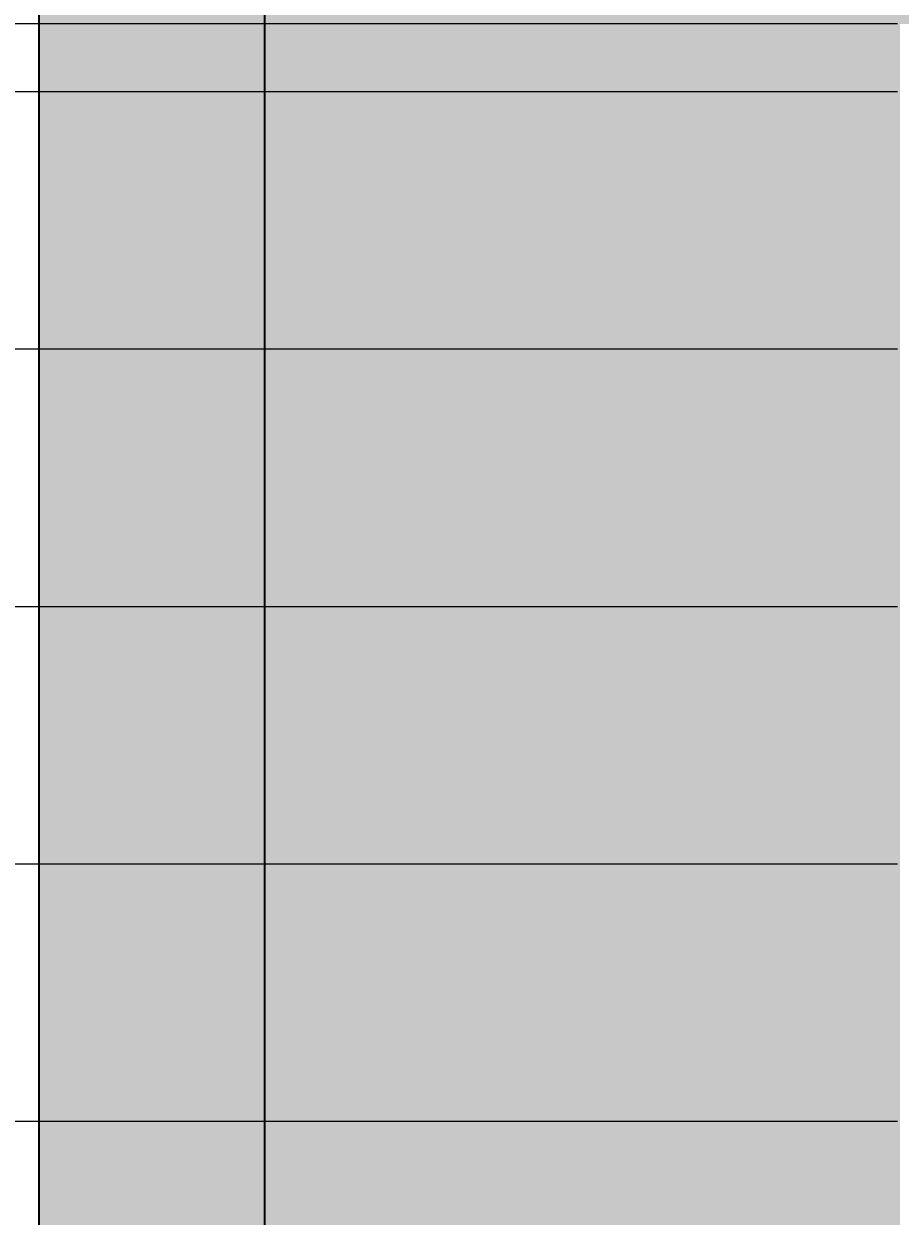
# Model space of a CAD drawing. Units: feet. Extents: x 2695 to 2912, y 795 to 1139.
# Tile 43 of 83: x 2710 to 2731, y 1020 to 1048. Entities that reach past the tile are written whole.
import ezdxf

# ---------------------------------------------------------------- set-up
doc = ezdxf.new("R2010")
doc.units = ezdxf.units.FT
for name, color, linetype, lineweight in [('A-ANNO-DIMS', 2, 'Continuous', 18), ('A-ELEV', 7, 'Continuous', 35), ('A-ELEV-PATT', 252, 'Continuous', 13)]:
    doc.layers.add(name, color=color, linetype=linetype, lineweight=lineweight)
doc.styles.get("Standard").update_dxf_attribs({"font": 'arial.ttf'})
doc.dimstyles.get("Standard").update_dxf_attribs({"dimtxt": 0.18, "dimasz": 0.18, "dimexe": 0.18, "dimexo": 0.0625, "dimgap": 0.09, "dimtad": 0, "dimtih": 1, "dimtoh": 1, "dimdec": 1, "dimzin": 0, "dimdsep": 46, "dimlunit": 3, "dimtxsty": 'Standard', "dimcen": 0.09, "dimadec": 0, "dimazin": 0, "dimtfac": 1, "dimtdec": 1, "dimtofl": 0, "dimtmove": 0, "dimatfit": 3, "dimfxl": 1, "dimtolj": 1, "dimtzin": 0, "dimarcsym": 0})

# ---------------------------------------------------------------- blocks, each defined once
blk = doc.blocks.new('*D12')
at = {"layer": 'A-ANNO-DIMS', "color": 0, "lineweight": -2, "transparency": 16777216}
for p, q in [((2710.574, 1122.931), (2694.681, 1122.931)), ((2694.861, 1122.751), (2694.861, 967.113)), ((2694.861, 811.111), (2694.861, 966.749)), ((2710.574, 810.931), (2694.681, 810.931))]:
    blk.add_line(p, q, dxfattribs=at)
at = {"layer": 'A-ANNO-DIMS', "color": 0, "transparency": 16777216}
for points in [[(2694.831, 1122.751), (2694.891, 1122.751), (2694.861, 1122.931)], [(2694.831, 811.111), (2694.891, 811.111), (2694.861, 810.931)]]:
    blk.add_solid(points, dxfattribs=at)
at = {"layer": 'Defpoints', "color": 0, "transparency": 16777216}
for p in [(2694.861, 1122.931), (2710.636, 1122.931), (2710.636, 810.931)]:
    blk.add_point(p, dxfattribs=at)
at = {"layer": 'A-ANNO-DIMS', "color": 0, "transparency": 16777216, "insert": (2694.861, 966.931), "char_height": 0.18, "attachment_point": 5}
blk.add_mtext('\\A1;312', dxfattribs=at)
blk = doc.blocks.new('*D41')
at = {"layer": 'A-ANNO-DIMS', "color": 0, "lineweight": -2, "transparency": 16777216}
for p, q in [((2730.646, 1022.518), (2694.681, 1022.518)), ((2694.861, 1022.338), (2694.861, 1019.7)), ((2694.861, 1016.698), (2694.861, 1019.336)), ((2730.646, 1016.518), (2694.681, 1016.518))]:
    blk.add_line(p, q, dxfattribs=at)
at = {"layer": 'A-ANNO-DIMS', "color": 0, "transparency": 16777216}
for points in [[(2694.831, 1022.338), (2694.891, 1022.338), (2694.861, 1022.518)], [(2694.831, 1016.698), (2694.891, 1016.698), (2694.861, 1016.518)]]:
    blk.add_solid(points, dxfattribs=at)
at = {"layer": 'Defpoints', "color": 0, "transparency": 16777216}
for p in [(2694.861, 1022.518), (2730.708, 1022.518), (2730.708, 1016.518)]:
    blk.add_point(p, dxfattribs=at)
at = {"layer": 'A-ANNO-DIMS', "color": 0, "transparency": 16777216, "insert": (2694.861, 1019.518), "char_height": 0.18, "attachment_point": 5}
blk.add_mtext('\\A1;6', dxfattribs=at)
blk = doc.blocks.new('*D42')
at = {"layer": 'A-ANNO-DIMS', "color": 0, "lineweight": -2, "transparency": 16777216}
for p, q in [((2730.646, 1028.518), (2694.681, 1028.518)), ((2694.861, 1028.338), (2694.861, 1025.7)), ((2694.861, 1022.698), (2694.861, 1025.336)), ((2730.646, 1022.518), (2694.681, 1022.518))]:
    blk.add_line(p, q, dxfattribs=at)
at = {"layer": 'A-ANNO-DIMS', "color": 0, "transparency": 16777216}
for points in [[(2694.831, 1028.338), (2694.891, 1028.338), (2694.861, 1028.518)], [(2694.831, 1022.698), (2694.891, 1022.698), (2694.861, 1022.518)]]:
    blk.add_solid(points, dxfattribs=at)
at = {"layer": 'Defpoints', "color": 0, "transparency": 16777216}
for p in [(2694.861, 1028.518), (2730.708, 1028.518), (2730.708, 1022.518)]:
    blk.add_point(p, dxfattribs=at)
at = {"layer": 'A-ANNO-DIMS', "color": 0, "transparency": 16777216, "insert": (2694.861, 1025.518), "char_height": 0.18, "attachment_point": 5}
blk.add_mtext('\\A1;6', dxfattribs=at)
blk = doc.blocks.new('*D43')
at = {"layer": 'A-ANNO-DIMS', "color": 0, "lineweight": -2, "transparency": 16777216}
for p, q in [((2730.646, 1034.518), (2694.681, 1034.518)), ((2694.861, 1034.338), (2694.861, 1031.7)), ((2694.861, 1028.698), (2694.861, 1031.336)), ((2730.646, 1028.518), (2694.681, 1028.518))]:
    blk.add_line(p, q, dxfattribs=at)
at = {"layer": 'A-ANNO-DIMS', "color": 0, "transparency": 16777216}
for points in [[(2694.831, 1034.338), (2694.891, 1034.338), (2694.861, 1034.518)], [(2694.831, 1028.698), (2694.891, 1028.698), (2694.861, 1028.518)]]:
    blk.add_solid(points, dxfattribs=at)
at = {"layer": 'Defpoints', "color": 0, "transparency": 16777216}
for p in [(2694.861, 1034.518), (2730.708, 1034.518), (2730.708, 1028.518)]:
    blk.add_point(p, dxfattribs=at)
at = {"layer": 'A-ANNO-DIMS', "color": 0, "transparency": 16777216, "insert": (2694.861, 1031.518), "char_height": 0.18, "attachment_point": 5}
blk.add_mtext('\\A1;6', dxfattribs=at)
blk = doc.blocks.new('*D44')
at = {"layer": 'A-ANNO-DIMS', "color": 0, "lineweight": -2, "transparency": 16777216}
for p, q in [((2730.646, 1040.518), (2694.681, 1040.518)), ((2694.861, 1040.338), (2694.861, 1037.7)), ((2694.861, 1034.698), (2694.861, 1037.336)), ((2730.646, 1034.518), (2694.681, 1034.518))]:
    blk.add_line(p, q, dxfattribs=at)
at = {"layer": 'A-ANNO-DIMS', "color": 0, "transparency": 16777216}
for points in [[(2694.831, 1040.338), (2694.891, 1040.338), (2694.861, 1040.518)], [(2694.831, 1034.698), (2694.891, 1034.698), (2694.861, 1034.518)]]:
    blk.add_solid(points, dxfattribs=at)
at = {"layer": 'Defpoints', "color": 0, "transparency": 16777216}
for p in [(2694.861, 1040.518), (2730.708, 1040.518), (2730.708, 1034.518)]:
    blk.add_point(p, dxfattribs=at)
at = {"layer": 'A-ANNO-DIMS', "color": 0, "transparency": 16777216, "insert": (2694.861, 1037.518), "char_height": 0.18, "attachment_point": 5}
blk.add_mtext('\\A1;6', dxfattribs=at)
blk = doc.blocks.new('*D45')
at = {"layer": 'A-ANNO-DIMS', "color": 0, "lineweight": -2, "transparency": 16777216}
for p, q in [((2730.646, 1046.518), (2694.681, 1046.518)), ((2694.861, 1046.338), (2694.861, 1043.7)), ((2694.861, 1040.698), (2694.861, 1043.336)), ((2730.646, 1040.518), (2694.681, 1040.518))]:
    blk.add_line(p, q, dxfattribs=at)
at = {"layer": 'A-ANNO-DIMS', "color": 0, "transparency": 16777216}
for points in [[(2694.831, 1046.338), (2694.891, 1046.338), (2694.861, 1046.518)], [(2694.831, 1040.698), (2694.891, 1040.698), (2694.861, 1040.518)]]:
    blk.add_solid(points, dxfattribs=at)
at = {"layer": 'Defpoints', "color": 0, "transparency": 16777216}
for p in [(2694.861, 1046.518), (2730.708, 1046.518), (2730.708, 1040.518)]:
    blk.add_point(p, dxfattribs=at)
at = {"layer": 'A-ANNO-DIMS', "color": 0, "transparency": 16777216, "insert": (2694.861, 1043.518), "char_height": 0.18, "attachment_point": 5}
blk.add_mtext('\\A1;6', dxfattribs=at)
blk = doc.blocks.new('*D46')
at = {"layer": 'A-ANNO-DIMS', "color": 0, "lineweight": -2, "transparency": 16777216}
for p, q in [((2730.646, 1048.105), (2694.681, 1048.105)), ((2694.861, 1047.925), (2694.861, 1047.493)), ((2694.861, 1046.698), (2694.861, 1047.13)), ((2730.646, 1046.518), (2694.681, 1046.518))]:
    blk.add_line(p, q, dxfattribs=at)
at = {"layer": 'A-ANNO-DIMS', "color": 0, "transparency": 16777216}
for points in [[(2694.831, 1047.925), (2694.891, 1047.925), (2694.861, 1048.105)], [(2694.831, 1046.698), (2694.891, 1046.698), (2694.861, 1046.518)]]:
    blk.add_solid(points, dxfattribs=at)
at = {"layer": 'Defpoints', "color": 0, "transparency": 16777216}
for p in [(2694.861, 1048.105), (2730.708, 1048.105), (2730.708, 1046.518)]:
    blk.add_point(p, dxfattribs=at)
at = {"layer": 'A-ANNO-DIMS', "color": 0, "transparency": 16777216, "insert": (2694.861, 1047.312), "char_height": 0.18, "attachment_point": 5}
blk.add_mtext('\\A1;1.59', dxfattribs=at)

msp = doc.modelspace()

# ---------------------------------------------------------------- hatches: boundary and pattern name
at = {"layer": 'A-ELEV-PATT'}
h = msp.add_hatch(color=256, dxfattribs=at)
h.set_gradient(color1=(255, 255, 255), tint=1)
h.paths.add_polyline_path([(2770.6361, 1122.9306), (2710.6361, 1122.9306), (2710.6361, 1118.4096), (2770.6361, 1118.4096)])
h.paths.add_polyline_path([(2890.6361, 1107.8588), (2770.6361, 1107.8588), (2770.6361, 1103.3378), (2890.6361, 1103.3378)])
h.paths.add_polyline_path([(2890.6361, 1062.9306), (2710.6361, 1062.9306), (2710.6361, 1056.9306), (2710.6361, 936.9306), (2710.6361, 924.3105), (2716.5358, 924.3105), (2890.6361, 924.3105), (2890.6361, 936.9306), (2715.8852, 936.9306), (2715.8852, 1050.3105), (2890.6361, 1050.3105)])
h.paths.add_polyline_path([(2716.5358, 924.3105), (2710.6361, 924.3105), (2710.6361, 810.9306), (2716.5358, 810.9306)])
h = msp.add_hatch(color=256, dxfattribs=at)
h.set_gradient(color1=(147, 149, 152), color2=(147, 149, 152), tint=1)
h.paths.add_polyline_path([(2770.6361, 1118.4096), (2710.6361, 1118.4096), (2710.6361, 1062.9306), (2770.6361, 1062.9306)])
h.paths.add_polyline_path([(2890.6361, 1103.3378), (2770.6361, 1103.3378), (2770.6361, 1062.9306), (2890.6361, 1062.9306)])
h.paths.add_polyline_path([(2730.7081, 1048.1052), (2755.1125, 1048.1052), (2755.1125, 936.9306), (2770.6361, 936.9306), (2770.6361, 1050.3105), (2715.8852, 1050.3105), (2715.8852, 936.9306), (2730.7081, 936.9306)])
h.paths.add_polyline_path([(2890.6361, 1050.3105), (2770.6361, 1050.3105), (2770.6361, 971.9673), (2778.0341, 971.9673), (2778.0341, 1020.8235), (2843.575, 1020.8235), (2843.575, 971.9673), (2890.6361, 971.9673)])
h.paths.add_polyline_path([(2888.1882, 970.7156), (2843.575, 970.7156), (2843.575, 964.8267), (2888.1882, 964.8267)])
h.paths.add_polyline_path([(2888.1882, 964.1328), (2843.575, 964.1328), (2843.575, 956.614), (2888.1882, 956.614)])
h.paths.add_polyline_path([(2888.1882, 955.9202), (2843.575, 955.9202), (2843.575, 949.2892), (2888.1882, 949.2892)])
h.paths.add_polyline_path([(2888.1882, 948.5954), (2843.575, 948.5954), (2843.575, 941.3507), (2888.1882, 941.3507)])
h.paths.add_polyline_path([(2888.1882, 940.6569), (2843.575, 940.6569), (2843.575, 936.9306), (2888.1882, 936.9306)])
h.paths.add_polyline_path([(2890.6361, 970.7156), (2888.9368, 970.7156), (2888.9368, 964.8267), (2890.6361, 964.8267)])
h.paths.add_polyline_path([(2890.6361, 964.1328), (2888.9368, 964.1328), (2888.9368, 956.614), (2890.6361, 956.614)])
h.paths.add_polyline_path([(2890.6361, 955.9202), (2888.9368, 955.9202), (2888.9368, 949.2892), (2890.6361, 949.2892)])
h.paths.add_polyline_path([(2890.6361, 940.6569), (2888.9368, 940.6569), (2888.9368, 936.9306), (2890.6361, 936.9306)])
h.paths.add_polyline_path([(2890.6361, 948.5954), (2888.9368, 948.5954), (2888.9368, 941.3507), (2890.6361, 941.3507)])
h.paths.add_polyline_path([(2772.5216, 970.7156), (2770.6361, 970.7156), (2770.6361, 964.8267), (2772.5216, 964.8267)])
h.paths.add_polyline_path([(2772.5216, 964.1328), (2770.6361, 964.1328), (2770.6361, 956.614), (2772.5216, 956.614)])
h.paths.add_polyline_path([(2772.5216, 955.9202), (2770.6361, 955.9202), (2770.6361, 949.2892), (2772.5216, 949.2892)])
h.paths.add_polyline_path([(2772.5216, 948.5954), (2770.6361, 948.5954), (2770.6361, 941.3507), (2772.5216, 941.3507)])
h.paths.add_polyline_path([(2772.5216, 940.6569), (2770.6361, 940.6569), (2770.6361, 936.9306), (2772.5216, 936.9306)])
h.paths.add_polyline_path([(2778.0341, 940.6569), (2773.2702, 940.6569), (2773.2702, 936.9306), (2778.0341, 936.9306)])
h.paths.add_polyline_path([(2778.0341, 970.7156), (2773.2702, 970.7156), (2773.2702, 964.8267), (2778.0341, 964.8267)])
h.paths.add_polyline_path([(2778.0341, 964.1328), (2773.2702, 964.1328), (2773.2702, 956.614), (2778.0341, 956.614)])
h.paths.add_polyline_path([(2778.0341, 955.9202), (2773.2702, 955.9202), (2773.2702, 949.2892), (2778.0341, 949.2892)])
h.paths.add_polyline_path([(2778.0341, 948.5954), (2773.2702, 948.5954), (2773.2702, 941.3507), (2778.0341, 941.3507)])
h.paths.add_polyline_path([(2810.0407, 940.6569), (2780.0341, 940.6569), (2780.0341, 936.9306), (2810.0407, 936.9306)])
h.paths.add_polyline_path([(2890.6361, 924.3105), (2770.6361, 924.3105), (2770.6361, 810.9306), (2773.5029, 810.9306), (2773.5029, 905.5143), (2805.9398, 905.5143), (2838.3767, 905.5143), (2838.3767, 810.9306), (2890.6361, 810.9306)])

# ---------------------------------------------------------------- linework, layer by layer
at = {"layer": 'A-ELEV'}
for p, q in [((2710.6361, 936.9306), (2710.6361, 1056.9306)), ((2715.8852, 1050.3105), (2715.8852, 936.9306))]:
    msp.add_line(p, q, dxfattribs=at)
msp.add_lwpolyline([(2715.8852, 1050.3105), (2715.8852, 936.9306)], dxfattribs=at)

# ---------------------------------------------------------------- dimensions: what is measured, and where the dimension line sits
at = {"layer": 'A-ANNO-DIMS'}
for base, p1, p2, override, picture, middle in [((2694.8611, 1122.9306), (2710.6361, 810.9306), (2710.6361, 1122.9306), {"dimdec": 0, "dimlfac": 1, "dimrnd": 0, "dimzin": 0, "dimdsep": 46, "dimlunit": 2}, '*D12', (2694.8611, 966.9306)), ((2694.8611, 1048.1052), (2730.7081, 1046.5179), (2730.7081, 1048.1052), {"dimdec": 2, "dimlfac": 1, "dimrnd": 0, "dimzin": 0, "dimdsep": 46, "dimlunit": 2}, '*D46', (2694.8611, 1047.3116)), ((2694.8611, 1046.5179), (2730.7081, 1040.5179), (2730.7081, 1046.5179), {"dimdec": 0, "dimlfac": 1, "dimrnd": 0, "dimzin": 0, "dimdsep": 46, "dimlunit": 2}, '*D45', (2694.8611, 1043.5179)), ((2694.8611, 1040.5179), (2730.7081, 1034.5179), (2730.7081, 1040.5179), {"dimdec": 0, "dimlfac": 1, "dimrnd": 0, "dimzin": 0, "dimdsep": 46, "dimlunit": 2}, '*D44', (2694.8611, 1037.5179)), ((2694.8611, 1034.5179), (2730.7081, 1028.5179), (2730.7081, 1034.5179), {"dimdec": 0, "dimlfac": 1, "dimrnd": 0, "dimzin": 0, "dimdsep": 46, "dimlunit": 2}, '*D43', (2694.8611, 1031.5179)), ((2694.8611, 1028.5179), (2730.7081, 1022.5179), (2730.7081, 1028.5179), {"dimdec": 0, "dimlfac": 1, "dimrnd": 0, "dimzin": 0, "dimdsep": 46, "dimlunit": 2}, '*D42', (2694.8611, 1025.5179)), ((2694.8611, 1022.5179), (2730.7081, 1016.5179), (2730.7081, 1022.5179), {"dimdec": 0, "dimlfac": 1, "dimrnd": 0, "dimzin": 0, "dimdsep": 46, "dimlunit": 2}, '*D41', (2694.8611, 1019.5179))]:
    dim = msp.add_linear_dim(base=base, p1=p1, p2=p2, angle=90, dimstyle='Standard', override=override, dxfattribs=at)
    dim.commit()
    dim.dimension.update_dxf_attribs({"geometry": picture, "text_midpoint": middle})

doc.saveas('drawing.dxf')
